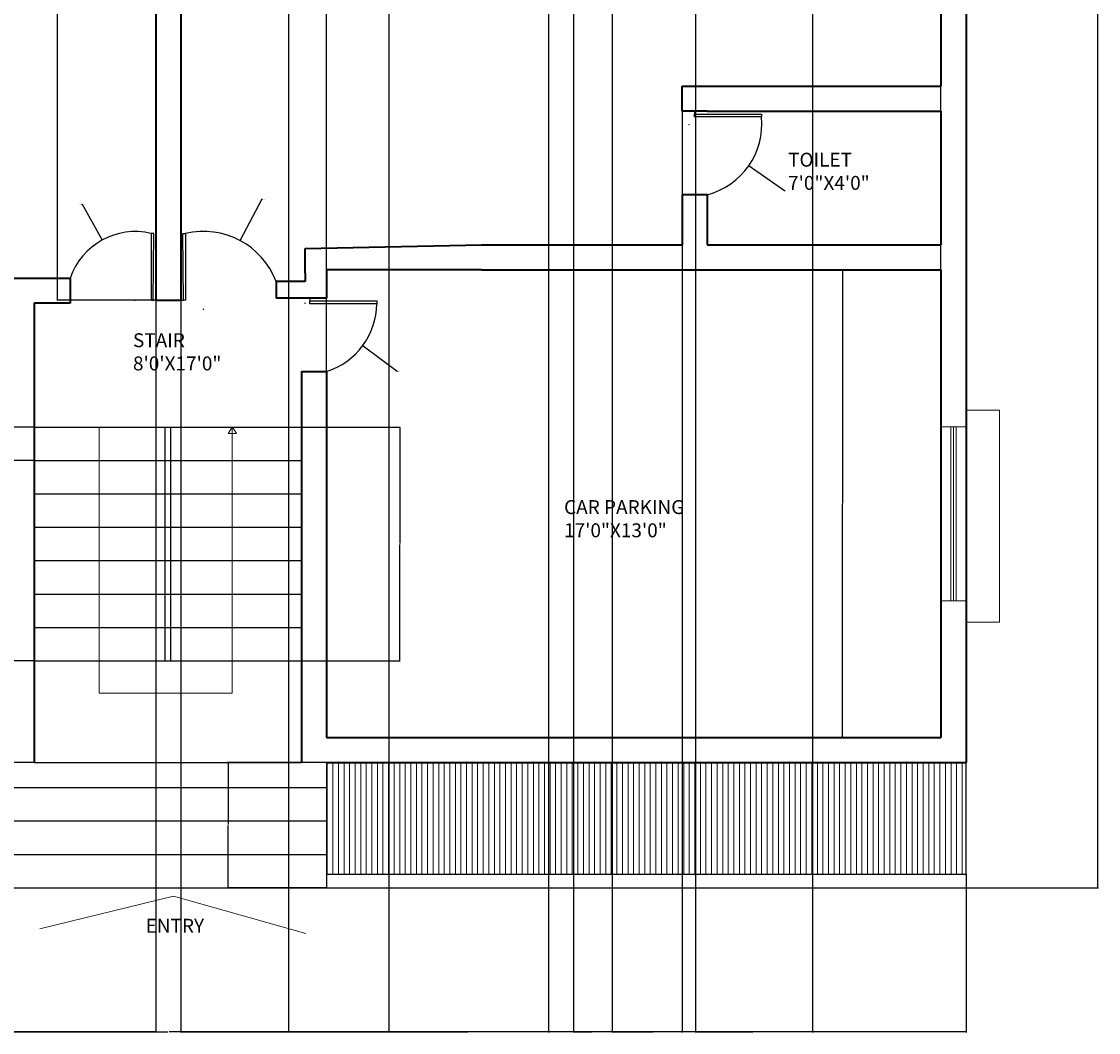
# Model space of a CAD drawing. Units: inches. Extents: x -35 to 633, y -653 to 119.
# Tile 2 of 4: x 246 to 633, y -653 to -289. Entities that reach past the tile are written whole.
import ezdxf

# ---------------------------------------------------------------- set-up
doc = ezdxf.new("R2010")
doc.units = ezdxf.units.IN
doc.header["$MEASUREMENT"] = 0
for name, color, linetype, lineweight in [('A-ANNO-DIMS', 2, 'Continuous', 18), ('A-ANNO-SYMB', 2, 'Continuous', 18), ('A-ANNO-TEXT', 7, 'Continuous', 25), ('A-AREA-IDEN', 7, 'Continuous', 18), ('A-DOOR', 3, 'Continuous', 25), ('A-FLOR-STRS', 7, 'Continuous', 25), ('A-GLAZ', 4, 'Continuous', 20), ('A-GLAZ-PROJ', 4, 'Continuous', 18), ('A-WALL', 7, 'Continuous', 35), ('L-HRDS', 8, 'Continuous', 25), ('L-HRDS-PATT', 252, 'Continuous', 13)]:
    doc.layers.add(name, color=color, linetype=linetype, lineweight=lineweight)
doc.styles.get("Standard").update_dxf_attribs({"font": 'arial.ttf'})
doc.dimstyles.get("Standard").update_dxf_attribs({"dimtxt": 0.18, "dimasz": 0.18, "dimexe": 0.18, "dimexo": 0.0625, "dimgap": 0.09, "dimtad": 0, "dimtih": 1, "dimtoh": 1, "dimdec": 4, "dimzin": 0, "dimdsep": 46, "dimtxsty": 'Standard', "dimcen": 0.09, "dimadec": 0, "dimazin": 0, "dimtfac": 1, "dimtdec": 4, "dimtofl": 0, "dimtmove": 0, "dimatfit": 3, "dimfxl": 1, "dimtolj": 1, "dimtzin": 0, "dimarcsym": 0})

# ---------------------------------------------------------------- blocks, each defined once
blk = doc.blocks.new('DOOR-LEAF-24IN')
for p, q in [((-1, 24), (-2, 24)), ((-2, 24), (-2, 0)), ((-1, 0), (-1, 24)), ((-2, 0), (-1, 0)), ((0, 0), (-1, 0))]:
    blk.add_line(p, q)
blk = doc.blocks.new('*D10')
at = {"layer": 'A-ANNO-DIMS', "color": 0, "lineweight": -2, "transparency": 16777216}
for p, q in [((12.69, -594.87), (12.69, -652.72)), ((585.69, -595.88), (585.69, -652.72)), ((12.87, -652.54), (298.9, -652.54)), ((585.51, -652.54), (299.48, -652.54))]:
    blk.add_line(p, q, dxfattribs=at)
at = {"layer": 'A-ANNO-DIMS', "color": 0, "transparency": 16777216}
for points in [[(12.87, -652.51), (12.87, -652.57), (12.69, -652.54)], [(585.51, -652.51), (585.51, -652.57), (585.69, -652.54)]]:
    blk.add_solid(points, dxfattribs=at)
at = {"layer": 'Defpoints', "color": 0, "transparency": 16777216}
for p in [(12.69, -594.81), (585.69, -595.82), (585.69, -652.54)]:
    blk.add_point(p, dxfattribs=at)
at = {"layer": 'A-ANNO-DIMS', "color": 0, "transparency": 16777216, "insert": (299.19, -652.54), "char_height": 0.18, "attachment_point": 5}
blk.add_mtext('\\A1;573', dxfattribs=at)
blk = doc.blocks.new('*D19')
at = {"layer": 'A-ANNO-DIMS', "color": 0, "lineweight": -2, "transparency": 16777216}
for p, q in [((303.69, 17.22), (303.69, -652.72)), ((342.39, 17.22), (342.39, -652.72)), ((303.87, -652.54), (322.57, -652.54)), ((342.21, -652.54), (323.5, -652.54))]:
    blk.add_line(p, q, dxfattribs=at)
at = {"layer": 'A-ANNO-DIMS', "color": 0, "transparency": 16777216}
for points in [[(303.87, -652.51), (303.87, -652.57), (303.69, -652.54)], [(342.21, -652.51), (342.21, -652.57), (342.39, -652.54)]]:
    blk.add_solid(points, dxfattribs=at)
at = {"layer": 'Defpoints', "color": 0, "transparency": 16777216}
for p in [(303.69, 17.29), (342.39, 17.29), (342.39, -652.54)]:
    blk.add_point(p, dxfattribs=at)
at = {"layer": 'A-ANNO-DIMS', "color": 0, "transparency": 16777216, "insert": (323.04, -652.54), "char_height": 0.18, "attachment_point": 5}
blk.add_mtext('\\A1;38.695', dxfattribs=at)
blk = doc.blocks.new('*D20')
at = {"layer": 'A-ANNO-DIMS', "color": 0, "lineweight": -2, "transparency": 16777216}
for p, q in [((378.39, 17.22), (378.39, -652.72)), ((435.69, 17.22), (435.69, -652.72)), ((378.57, -652.54), (406.71, -652.54)), ((435.51, -652.54), (407.36, -652.54))]:
    blk.add_line(p, q, dxfattribs=at)
at = {"layer": 'A-ANNO-DIMS', "color": 0, "transparency": 16777216}
for points in [[(378.57, -652.51), (378.57, -652.57), (378.39, -652.54)], [(435.51, -652.51), (435.51, -652.57), (435.69, -652.54)]]:
    blk.add_solid(points, dxfattribs=at)
at = {"layer": 'Defpoints', "color": 0, "transparency": 16777216}
for p in [(378.39, 17.29), (435.69, 17.29), (435.69, -652.54)]:
    blk.add_point(p, dxfattribs=at)
at = {"layer": 'A-ANNO-DIMS', "color": 0, "transparency": 16777216, "insert": (407.04, -652.54), "char_height": 0.18, "attachment_point": 5}
blk.add_mtext('\\A1;57.3', dxfattribs=at)
blk = doc.blocks.new('*D21')
at = {"layer": 'A-ANNO-DIMS', "color": 0, "lineweight": -2, "transparency": 16777216}
for p, q in [((444.69, 17.22), (444.69, -652.72)), ((458.58, 17.22), (458.58, -652.72)), ((444.87, -652.54), (451.25, -652.54)), ((458.4, -652.54), (452.02, -652.54))]:
    blk.add_line(p, q, dxfattribs=at)
at = {"layer": 'A-ANNO-DIMS', "color": 0, "transparency": 16777216}
for points in [[(444.87, -652.51), (444.87, -652.57), (444.69, -652.54)], [(458.4, -652.51), (458.4, -652.57), (458.58, -652.54)]]:
    blk.add_solid(points, dxfattribs=at)
at = {"layer": 'Defpoints', "color": 0, "transparency": 16777216}
for p in [(444.69, 17.29), (458.58, 17.29), (458.58, -652.54)]:
    blk.add_point(p, dxfattribs=at)
at = {"layer": 'A-ANNO-DIMS', "color": 0, "transparency": 16777216, "insert": (451.64, -652.54), "char_height": 0.18, "attachment_point": 5}
blk.add_mtext('\\A1;13.89', dxfattribs=at)
blk = doc.blocks.new('*D22')
at = {"layer": 'A-ANNO-DIMS', "color": 0, "lineweight": -2, "transparency": 16777216}
for p, q in [((458.58, 17.22), (458.58, -652.72)), ((488.58, 17.22), (488.58, -652.72)), ((458.76, -652.54), (473.36, -652.54)), ((488.4, -652.54), (473.8, -652.54))]:
    blk.add_line(p, q, dxfattribs=at)
at = {"layer": 'A-ANNO-DIMS', "color": 0, "transparency": 16777216}
for points in [[(458.76, -652.51), (458.76, -652.57), (458.58, -652.54)], [(488.4, -652.51), (488.4, -652.57), (488.58, -652.54)]]:
    blk.add_solid(points, dxfattribs=at)
at = {"layer": 'Defpoints', "color": 0, "transparency": 16777216}
for p in [(458.58, 17.29), (488.58, 17.29), (488.58, -652.54)]:
    blk.add_point(p, dxfattribs=at)
at = {"layer": 'A-ANNO-DIMS', "color": 0, "transparency": 16777216, "insert": (473.58, -652.54), "char_height": 0.18, "attachment_point": 5}
blk.add_mtext('\\A1;30', dxfattribs=at)
blk = doc.blocks.new('*D23')
at = {"layer": 'A-ANNO-DIMS', "color": 0, "lineweight": -2, "transparency": 16777216}
for p, q in [((488.58, 17.22), (488.58, -652.72)), ((530.49, 17.22), (530.49, -652.72)), ((488.76, -652.54), (509.15, -652.54)), ((530.31, -652.54), (509.91, -652.54))]:
    blk.add_line(p, q, dxfattribs=at)
at = {"layer": 'A-ANNO-DIMS', "color": 0, "transparency": 16777216}
for points in [[(488.76, -652.51), (488.76, -652.57), (488.58, -652.54)], [(530.31, -652.51), (530.31, -652.57), (530.49, -652.54)]]:
    blk.add_solid(points, dxfattribs=at)
at = {"layer": 'Defpoints', "color": 0, "transparency": 16777216}
for p in [(488.58, 17.29), (530.49, 17.29), (530.49, -652.54)]:
    blk.add_point(p, dxfattribs=at)
at = {"layer": 'A-ANNO-DIMS', "color": 0, "transparency": 16777216, "insert": (509.53, -652.54), "char_height": 0.18, "attachment_point": 5}
blk.add_mtext('\\A1;41.91', dxfattribs=at)
blk = doc.blocks.new('*D24')
at = {"layer": 'A-ANNO-DIMS', "color": 0, "lineweight": -2, "transparency": 16777216}
for p, q in [((585.75, 83.29), (633.22, 83.29)), ((633.04, 83.11), (633.04, -258.53)), ((633.04, -600.53), (633.04, -258.89)), ((356.04, -600.71), (633.22, -600.71))]:
    blk.add_line(p, q, dxfattribs=at)
at = {"layer": 'A-ANNO-DIMS', "color": 0, "transparency": 16777216}
for points in [[(633.01, 83.11), (633.07, 83.11), (633.04, 83.29)], [(633.01, -600.53), (633.07, -600.53), (633.04, -600.71)]]:
    blk.add_solid(points, dxfattribs=at)
at = {"layer": 'Defpoints', "color": 0, "transparency": 16777216}
for p in [(585.69, 83.29), (355.98, -600.71), (633.04, -600.71)]:
    blk.add_point(p, dxfattribs=at)
at = {"layer": 'A-ANNO-DIMS', "color": 0, "transparency": 16777216, "insert": (633.04, -258.71), "char_height": 0.18, "attachment_point": 5}
blk.add_mtext('\\A1;684', dxfattribs=at)
blk = doc.blocks.new('*D37')
at = {"layer": 'A-ANNO-DIMS', "color": 0, "lineweight": -2, "transparency": 16777216}
for p, q in [((355.98, -546.65), (355.98, 118.82)), ((356.16, 118.64), (465.94, 118.64)), ((576.51, 118.64), (466.73, 118.64)), ((576.69, -546.65), (576.69, 118.82))]:
    blk.add_line(p, q, dxfattribs=at)
at = {"layer": 'A-ANNO-DIMS', "color": 0, "transparency": 16777216}
for points in [[(356.16, 118.67), (356.16, 118.61), (355.98, 118.64)], [(576.51, 118.67), (576.51, 118.61), (576.69, 118.64)]]:
    blk.add_solid(points, dxfattribs=at)
at = {"layer": 'Defpoints', "color": 0, "transparency": 16777216}
for p in [(576.69, 118.64), (355.98, -546.71), (576.69, -546.71)]:
    blk.add_point(p, dxfattribs=at)
at = {"layer": 'A-ANNO-DIMS', "color": 0, "transparency": 16777216, "insert": (466.33, 118.64), "char_height": 0.18, "attachment_point": 5}
blk.add_mtext('\\A1;220.7', dxfattribs=at)
blk = doc.blocks.new('*D40')
at = {"layer": 'A-ANNO-DIMS', "color": 0, "lineweight": -2, "transparency": 16777216}
for p, q in [((576.63, -378.71), (541.16, -378.71)), ((541.34, -378.89), (541.34, -462.53)), ((541.34, -546.53), (541.34, -462.89)), ((576.63, -546.71), (541.16, -546.71))]:
    blk.add_line(p, q, dxfattribs=at)
at = {"layer": 'A-ANNO-DIMS', "color": 0, "transparency": 16777216}
for points in [[(541.31, -378.89), (541.37, -378.89), (541.34, -378.71)], [(541.31, -546.53), (541.37, -546.53), (541.34, -546.71)]]:
    blk.add_solid(points, dxfattribs=at)
at = {"layer": 'Defpoints', "color": 0, "transparency": 16777216}
for p in [(541.34, -378.71), (576.69, -378.71), (576.69, -546.71)]:
    blk.add_point(p, dxfattribs=at)
at = {"layer": 'A-ANNO-DIMS', "color": 0, "transparency": 16777216, "insert": (541.34, -462.71), "char_height": 0.18, "attachment_point": 5}
blk.add_mtext('\\A1;168', dxfattribs=at)
blk = doc.blocks.new('*D41')
at = {"layer": 'A-ANNO-DIMS', "color": 0, "lineweight": -2, "transparency": 16777216}
for p, q in [((347.04, -435.17), (382.51, -435.17)), ((382.33, -435.35), (382.33, -476.99)), ((382.33, -518.99), (382.33, -477.35)), ((347.04, -519.17), (382.51, -519.17))]:
    blk.add_line(p, q, dxfattribs=at)
at = {"layer": 'A-ANNO-DIMS', "color": 0, "transparency": 16777216}
for points in [[(382.3, -435.35), (382.36, -435.35), (382.33, -435.17)], [(382.3, -518.99), (382.36, -518.99), (382.33, -519.17)]]:
    blk.add_solid(points, dxfattribs=at)
at = {"layer": 'Defpoints', "color": 0, "transparency": 16777216}
for p in [(346.98, -435.17), (346.98, -519.17), (382.33, -519.17)]:
    blk.add_point(p, dxfattribs=at)
at = {"layer": 'A-ANNO-DIMS', "color": 0, "transparency": 16777216, "insert": (382.33, -477.17), "char_height": 0.18, "attachment_point": 5}
blk.add_mtext('\\A1;84', dxfattribs=at)
blk = doc.blocks.new('*D42')
at = {"layer": 'A-ANNO-DIMS', "color": 0, "lineweight": -2, "transparency": 16777216}
for p, q in [((250.91, -435.17), (215.45, -435.17)), ((215.63, -435.35), (215.63, -440.99)), ((215.63, -446.99), (215.63, -441.35)), ((250.91, -447.17), (215.45, -447.17))]:
    blk.add_line(p, q, dxfattribs=at)
at = {"layer": 'A-ANNO-DIMS', "color": 0, "transparency": 16777216}
for points in [[(215.6, -435.35), (215.66, -435.35), (215.63, -435.17)], [(215.6, -446.99), (215.66, -446.99), (215.63, -447.17)]]:
    blk.add_solid(points, dxfattribs=at)
at = {"layer": 'Defpoints', "color": 0, "transparency": 16777216}
for p in [(215.63, -435.17), (250.98, -435.17), (250.98, -447.17)]:
    blk.add_point(p, dxfattribs=at)
at = {"layer": 'A-ANNO-DIMS', "color": 0, "transparency": 16777216, "insert": (215.63, -441.17), "char_height": 0.18, "attachment_point": 5}
blk.add_mtext('\\A1;12', dxfattribs=at)
blk = doc.blocks.new('*D43')
at = {"layer": 'A-ANNO-DIMS', "color": 0, "lineweight": -2, "transparency": 16777216}
for p, q in [((250.91, -519.17), (215.45, -519.17)), ((215.63, -519.35), (215.63, -537.26)), ((215.63, -555.53), (215.63, -537.62)), ((250.91, -555.71), (215.45, -555.71))]:
    blk.add_line(p, q, dxfattribs=at)
at = {"layer": 'A-ANNO-DIMS', "color": 0, "transparency": 16777216}
for points in [[(215.6, -519.35), (215.66, -519.35), (215.63, -519.17)], [(215.6, -555.53), (215.66, -555.53), (215.63, -555.71)]]:
    blk.add_solid(points, dxfattribs=at)
at = {"layer": 'Defpoints', "color": 0, "transparency": 16777216}
for p in [(215.63, -519.17), (250.98, -519.17), (250.98, -555.71)]:
    blk.add_point(p, dxfattribs=at)
at = {"layer": 'A-ANNO-DIMS', "color": 0, "transparency": 16777216, "insert": (215.63, -537.44), "char_height": 0.18, "attachment_point": 5}
blk.add_mtext('\\A1;36.54', dxfattribs=at)
blk = doc.blocks.new('*D44')
at = {"layer": 'A-ANNO-DIMS', "color": 0, "lineweight": -2, "transparency": 16777216}
for p, q in [((355.91, -555.71), (320.45, -555.71)), ((320.63, -555.89), (320.63, -578.03)), ((320.63, -600.53), (320.63, -578.39)), ((355.91, -600.71), (320.45, -600.71))]:
    blk.add_line(p, q, dxfattribs=at)
at = {"layer": 'A-ANNO-DIMS', "color": 0, "transparency": 16777216}
for points in [[(320.6, -555.89), (320.66, -555.89), (320.63, -555.71)], [(320.6, -600.53), (320.66, -600.53), (320.63, -600.71)]]:
    blk.add_solid(points, dxfattribs=at)
at = {"layer": 'Defpoints', "color": 0, "transparency": 16777216}
for p in [(320.63, -555.71), (355.98, -555.71), (355.98, -600.71)]:
    blk.add_point(p, dxfattribs=at)
at = {"layer": 'A-ANNO-DIMS', "color": 0, "transparency": 16777216, "insert": (320.63, -578.21), "char_height": 0.18, "attachment_point": 5}
blk.add_mtext('\\A1;45', dxfattribs=at)
blk = doc.blocks.new('*D46')
at = {"layer": 'A-ANNO-DIMS', "color": 0, "lineweight": -2, "transparency": 16777216}
for p, q in [((294.63, -123.71), (259.16, -123.71)), ((259.34, -123.89), (259.34, -256.48)), ((259.34, -389.42), (259.34, -256.84)), ((294.63, -389.6), (259.16, -389.6))]:
    blk.add_line(p, q, dxfattribs=at)
at = {"layer": 'A-ANNO-DIMS', "color": 0, "transparency": 16777216}
for points in [[(259.31, -123.89), (259.37, -123.89), (259.34, -123.71)], [(259.31, -389.42), (259.37, -389.42), (259.34, -389.6)]]:
    blk.add_solid(points, dxfattribs=at)
at = {"layer": 'Defpoints', "color": 0, "transparency": 16777216}
for p in [(259.34, -123.71), (294.69, -123.71), (294.69, -389.6)]:
    blk.add_point(p, dxfattribs=at)
at = {"layer": 'A-ANNO-DIMS', "color": 0, "transparency": 16777216, "insert": (259.34, -256.66), "char_height": 0.18, "attachment_point": 5}
blk.add_mtext('\\A1;265.9', dxfattribs=at)
blk = doc.blocks.new('*D47')
at = {"layer": 'A-ANNO-DIMS', "color": 0, "lineweight": -2, "transparency": 16777216}
for p, q in [((294.69, -123.78), (294.69, -652.72)), ((126.69, -312.78), (126.69, -652.72)), ((126.87, -652.54), (210.41, -652.54)), ((294.51, -652.54), (210.97, -652.54))]:
    blk.add_line(p, q, dxfattribs=at)
at = {"layer": 'A-ANNO-DIMS', "color": 0, "transparency": 16777216}
for points in [[(126.87, -652.51), (126.87, -652.57), (126.69, -652.54)], [(294.51, -652.51), (294.51, -652.57), (294.69, -652.54)]]:
    blk.add_solid(points, dxfattribs=at)
at = {"layer": 'Defpoints', "color": 0, "transparency": 16777216}
for p in [(294.69, -123.71), (126.69, -312.71), (294.69, -652.54)]:
    blk.add_point(p, dxfattribs=at)
at = {"layer": 'A-ANNO-DIMS', "color": 0, "transparency": 16777216, "insert": (210.69, -652.54), "char_height": 0.18, "attachment_point": 5}
blk.add_mtext('\\A1;168', dxfattribs=at)
blk = doc.blocks.new('*D48')
at = {"layer": 'A-ANNO-DIMS', "color": 0, "lineweight": -2, "transparency": 16777216}
for p, q in [((303.69, -123.78), (303.69, -652.72)), ((483.69, -312.78), (483.69, -652.72)), ((303.87, -652.54), (393.41, -652.54)), ((483.51, -652.54), (393.97, -652.54))]:
    blk.add_line(p, q, dxfattribs=at)
at = {"layer": 'A-ANNO-DIMS', "color": 0, "transparency": 16777216}
for points in [[(303.87, -652.51), (303.87, -652.57), (303.69, -652.54)], [(483.51, -652.51), (483.51, -652.57), (483.69, -652.54)]]:
    blk.add_solid(points, dxfattribs=at)
at = {"layer": 'Defpoints', "color": 0, "transparency": 16777216}
for p in [(303.69, -123.71), (483.69, -312.71), (483.69, -652.54)]:
    blk.add_point(p, dxfattribs=at)
at = {"layer": 'A-ANNO-DIMS', "color": 0, "transparency": 16777216, "insert": (393.69, -652.54), "char_height": 0.18, "attachment_point": 5}
blk.add_mtext('\\A1;180', dxfattribs=at)
blk = doc.blocks.new('*D54')
at = {"layer": 'A-ANNO-DIMS', "color": 0, "lineweight": -2, "transparency": 16777216}
for p, q in [((332.74, -353.35), (324.98, -367.99)), ((332.92, -353.35), (332.74, -353.35)), ((311.71, -392.81), (311.89, -392.81)), ((311.8, -392.9), (311.8, -392.72))]:
    blk.add_line(p, q, dxfattribs=at)
at = {"layer": 'A-ANNO-DIMS', "color": 0, "transparency": 16777216}
blk.add_solid([(324.95, -367.97), (325, -368), (324.89, -368.15)], dxfattribs=at)
at = {"layer": 'Defpoints', "color": 0, "transparency": 16777216}
for p in [(324.89, -368.15), (311.8, -392.81)]:
    blk.add_point(p, dxfattribs=at)
at = {"layer": 'A-ANNO-DIMS', "color": 0, "transparency": 16777216, "insert": (333.4, -353.35), "char_height": 0.18, "attachment_point": 5}
blk.add_mtext('\\A1;R27.92', dxfattribs=at)
blk = doc.blocks.new('*D56')
at = {"layer": 'A-ANNO-DIMS', "color": 0, "lineweight": -2, "transparency": 16777216}
for p, q in [((486.12, -326.41), (486.3, -326.41)), ((486.21, -326.5), (486.21, -326.32)), ((520.51, -350.29), (507.79, -341.44)), ((520.69, -350.29), (520.51, -350.29))]:
    blk.add_line(p, q, dxfattribs=at)
at = {"layer": 'A-ANNO-DIMS', "color": 0, "transparency": 16777216}
blk.add_solid([(507.81, -341.41), (507.77, -341.46), (507.64, -341.34)], dxfattribs=at)
at = {"layer": 'Defpoints', "color": 0, "transparency": 16777216}
for p in [(486.21, -326.41), (507.64, -341.34)]:
    blk.add_point(p, dxfattribs=at)
at = {"layer": 'A-ANNO-DIMS', "color": 0, "transparency": 16777216, "insert": (521.24, -350.29), "char_height": 0.18, "attachment_point": 5}
blk.add_mtext('\\A1;R26.125', dxfattribs=at)
blk = doc.blocks.new('*D57')
at = {"layer": 'A-ANNO-DIMS', "color": 0, "lineweight": -2, "transparency": 16777216}
for p, q in [((348.35, -390.76), (348.35, -390.58)), ((348.26, -390.67), (348.44, -390.67)), ((381.36, -415.19), (369.13, -406.11)), ((381.54, -415.19), (381.36, -415.19))]:
    blk.add_line(p, q, dxfattribs=at)
at = {"layer": 'A-ANNO-DIMS', "color": 0, "transparency": 16777216}
blk.add_solid([(369.15, -406.08), (369.11, -406.13), (368.98, -406)], dxfattribs=at)
at = {"layer": 'Defpoints', "color": 0, "transparency": 16777216}
for p in [(348.35, -390.67), (368.98, -406)]:
    blk.add_point(p, dxfattribs=at)
at = {"layer": 'A-ANNO-DIMS', "color": 0, "transparency": 16777216, "insert": (381.95, -415.19), "char_height": 0.18, "attachment_point": 5}
blk.add_mtext('\\A1;R25.7', dxfattribs=at)
blk = doc.blocks.new('*D59')
at = {"layer": 'A-ANNO-DIMS', "color": 0, "lineweight": -2, "transparency": 16777216}
for p, q in [((268.03, -355.09), (268.21, -355.09)), ((268.21, -355.09), (275.28, -367.85)), ((287.21, -389.55), (287.39, -389.55)), ((287.3, -389.64), (287.3, -389.46))]:
    blk.add_line(p, q, dxfattribs=at)
at = {"layer": 'A-ANNO-DIMS', "color": 0, "transparency": 16777216}
blk.add_solid([(275.31, -367.84), (275.26, -367.87), (275.37, -368.01)], dxfattribs=at)
at = {"layer": 'Defpoints', "color": 0, "transparency": 16777216}
for p in [(275.37, -368.01), (287.3, -389.55)]:
    blk.add_point(p, dxfattribs=at)
at = {"layer": 'A-ANNO-DIMS', "color": 0, "transparency": 16777216, "insert": (267.55, -355.09), "char_height": 0.18, "attachment_point": 5}
blk.add_mtext('\\A1;R24.62', dxfattribs=at)

msp = doc.modelspace()

# ---------------------------------------------------------------- hatches: boundary and pattern name
at = {"layer": 'L-HRDS-PATT'}
h = msp.add_hatch(dxfattribs=at)
h.set_pattern_fill('ANSI31', color=256, scale=16, angle=45, style=0)
h.set_pattern_definition([(90, (-2179.7136, -1471.1113), (-2, 0), [])])
h.paths.add_polyline_path([(355.9768, -595.8152), (585.6907, -595.8152), (585.6907, -555.713), (355.9768, -555.713)])

# ---------------------------------------------------------------- linework, layer by layer
at = {"layer": 'A-ANNO-SYMB'}
for p, q in [((274.3662, -435.1709), (274.3662, -530.8377)), ((322.0837, -435.1709), (320.7222, -437.529)), ((322.0837, -530.8377), (322.0837, -435.1709)), ((323.6397, -437.529), (322.2782, -435.1709)), ((320.7222, -437.529), (323.6397, -437.529)), ((274.3662, -530.8377), (322.0837, -530.8377)), ((301.0168, -603.7011), (253.0683, -615.458)), ((301.0168, -603.7011), (348.619, -617.187))]:
    msp.add_line(p, q, dxfattribs=at)
at = {"layer": 'A-DOOR'}
for p, q in [((294.0401, -365.606), (293.0401, -365.606)), ((293.0401, -365.606), (293.0401, -389.606)), ((293.6907, -389.6034), (294.0401, -365.606)), ((304.69, -389.6389), (304.3725, -365.641)), ((304.3725, -365.641), (305.3725, -365.641)), ((305.3725, -365.641), (305.3725, -389.641)), ((293.0401, -389.606), (294.0401, -389.606)), ((294.6907, -389.6034), (293.6907, -389.6034)), ((303.6907, -389.6034), (304.69, -389.6389)), ((305.3725, -389.641), (304.3725, -389.641))]:
    msp.add_line(p, q, dxfattribs=at)
for centre, radius, start, end in [((486.2053, -326.4062), 26.1246, 284.373894, 5.917194), ((287.2987, -389.5486), 24.6214, 76.515385, 161.44307), ((311.8045, -392.8103), 27.9203, 20.775692, 103.319004), ((348.3486, -390.6748), 25.7021, 287.265117, 359.542731)]:
    msp.add_arc(centre, radius, start, end, dxfattribs=at)
at = {"layer": 'A-FLOR-STRS'}
for p, q in [((250.9768, -435.1709), (346.9768, -435.1709)), ((297.9768, -435.1709), (297.9768, -519.1709)), ((299.9768, -435.1709), (299.9768, -519.1709)), ((250.9768, -447.1709), (346.9768, -447.1709)), ((250.9768, -459.1709), (346.9768, -459.1709)), ((250.9768, -471.1709), (346.9768, -471.1709)), ((250.9768, -483.1709), (346.9768, -483.1709)), ((250.9768, -495.1709), (346.9768, -495.1709)), ((250.9768, -507.1709), (346.9768, -507.1709)), ((250.9768, -507.1709), (346.9768, -507.1709)), ((250.9768, -519.1709), (346.9768, -519.1709)), ((250.9768, -555.713), (346.9768, -555.713)), ((355.9768, -555.713), (355.9768, -564.713)), ((241.9768, -564.713), (355.9768, -564.713)), ((355.9768, -564.713), (355.9768, -600.713)), ((241.9768, -576.713), (355.9768, -576.713)), ((241.9768, -588.713), (355.9768, -588.713)), ((241.9768, -600.713), (355.9768, -600.713)), ((254.4542, -600.713), (339.8944, -600.713))]:
    msp.add_line(p, q, dxfattribs=at)
at = {"layer": 'A-GLAZ'}
for p, q in [((576.6907, -435.0596), (585.6907, -435.0596)), ((580.1907, -435.0596), (580.1907, -497.5918)), ((581.1907, -435.0596), (581.1907, -497.5918)), ((582.1907, -435.0596), (582.1907, -497.5918)), ((576.6907, -497.5918), (585.6907, -497.5918))]:
    msp.add_line(p, q, dxfattribs=at)
at = {"layer": 'A-GLAZ-PROJ'}
for p, q in [((585.6907, -429.0928), (597.6907, -429.0928)), ((597.6907, -429.0928), (597.6907, -505.268)), ((597.6907, -505.268), (585.6907, -505.268))]:
    msp.add_line(p, q, dxfattribs=at)
at = {"layer": 'A-WALL'}
for p, q in [((585.6907, -114.713), (585.6907, -555.713)), ((294.6907, -123.713), (294.6907, -389.6034)), ((303.6907, -123.713), (303.6907, -389.6034)), ((576.6907, -180.713), (576.6907, -312.713)), ((483.6907, -312.713), (576.6907, -312.713)), ((483.6907, -321.713), (483.6907, -312.713)), ((492.6907, -321.713), (483.6907, -321.713)), ((492.6907, -321.713), (576.6907, -321.713)), ((576.6907, -321.713), (576.6907, -369.713)), ((483.6907, -351.713), (483.6907, -369.713)), ((492.6907, -351.713), (483.6907, -351.713)), ((492.6907, -351.713), (492.6907, -369.713)), ((348.3577, -370.9894), (411.6907, -369.713)), ((348.3577, -379.9347), (348.3577, -370.9894)), ((411.6907, -369.713), (483.6907, -369.713)), ((492.6907, -369.713), (576.6907, -369.713)), ((411.6907, -378.713), (355.9768, -378.713)), ((355.9768, -378.713), (355.9768, -388.88)), ((411.6907, -378.713), (576.6907, -378.713)), ((576.6907, -378.713), (576.6907, -546.713)), ((241.9768, -381.713), (250.9768, -381.713)), ((250.9768, -381.713), (263.9575, -381.713)), ((263.9575, -381.713), (263.9575, -390.713)), ((348.3577, -379.9347), (348.3577, -382.9067)), ((348.3577, -382.9067), (337.9094, -382.9067)), ((337.9094, -382.9067), (337.9094, -388.88)), ((294.6907, -389.6034), (303.6907, -389.6034)), ((355.9768, -388.88), (337.9094, -388.88)), ((250.9768, -390.713), (250.9768, -555.713)), ((263.9575, -390.713), (250.9768, -390.713)), ((346.9768, -415.2188), (346.9768, -555.713)), ((346.9768, -415.2188), (355.9768, -415.2188)), ((355.9768, -415.2188), (355.9768, -546.713)), ((355.9768, -546.713), (411.6907, -546.713)), ((411.6907, -546.713), (576.6907, -546.713)), ((355.9768, -555.713), (585.6907, -555.713))]:
    msp.add_line(p, q, dxfattribs=at)
at = {"layer": 'L-HRDS'}
for p, q in [((585.6907, -595.8152), (585.6907, -555.713)), ((355.9768, -595.8152), (585.6907, -595.8152))]:
    msp.add_line(p, q, dxfattribs=at)

# ---------------------------------------------------------------- block references
at = {"layer": 'A-DOOR', "extrusion": (0, 0, -1), "zscale": -1}
for p, rotation in [((-488.1907, -321.713), 89.99999999999999), ((-350.0498, -388.88), 90.00000000000003)]:
    msp.add_blockref('DOOR-LEAF-24IN', p, dxfattribs=dict(at, rotation=rotation))

# ---------------------------------------------------------------- texts
at = {"layer": 'A-ANNO-TEXT', "insert": (291.0525, -611.8649), "char_height": 5, "attachment_point": 1}
msp.add_mtext_dynamic_manual_height_columns('ENTRY', width=25.222092, gutter_width=25, heights=[0], dxfattribs=at)
at = {"layer": 'A-AREA-IDEN', "char_height": 5, "attachment_point": 1}
for s, width, insert in [('TOILET\\P7\'0"X4\'0"', 36.076101, (521.7779, -336.6165)), ('STAIR\\P8\'0\'X17\'0"', 41.424204, (286.4952, -401.4872)), ('CAR PARKING\\P17\'0"X13\'0"', 89.571033, (441.318, -461.447))]:
    msp.add_mtext_dynamic_manual_height_columns(s, width=width, gutter_width=25, heights=[0], dxfattribs=dict(at, insert=insert))

# ---------------------------------------------------------------- dimensions: what is measured, and where the dimension line sits
at = {"layer": 'A-ANNO-DIMS'}
for base, p1, p2, override, picture, middle in [((576.6907, 118.637), (355.9768, -546.713), (576.6907, -546.713), {"dimdec": 1, "dimlfac": 1, "dimrnd": 0, "dimzin": 0, "dimdsep": 46, "dimlunit": 2}, '*D37', (466.3337, 118.637)), ((342.3856, -652.537), (303.6907, 17.287), (342.3856, 17.287), {"dimdec": 3, "dimlfac": 1, "dimrnd": 0, "dimzin": 0, "dimdsep": 46, "dimlunit": 2}, '*D19', (323.0381, -652.537)), ((435.6907, -652.537), (378.3856, 17.287), (435.6907, 17.287), {"dimdec": 1, "dimlfac": 1, "dimrnd": 0, "dimzin": 0, "dimdsep": 46, "dimlunit": 2}, '*D20', (407.0381, -652.537)), ((458.5795, -652.537), (444.6907, 17.287), (458.5795, 17.287), {"dimdec": 2, "dimlfac": 1, "dimrnd": 0, "dimzin": 0, "dimdsep": 46, "dimlunit": 2}, '*D21', (451.6351, -652.537)), ((488.5795, -652.537), (458.5795, 17.287), (488.5795, 17.287), {"dimdec": 0, "dimlfac": 1, "dimrnd": 0, "dimzin": 0, "dimdsep": 46, "dimlunit": 2}, '*D22', (473.5795, -652.537)), ((530.4897, -652.537), (488.5795, 17.287), (530.4897, 17.287), {"dimdec": 2, "dimlfac": 1, "dimrnd": 0, "dimzin": 0, "dimdsep": 46, "dimlunit": 2}, '*D23', (509.5346, -652.537)), ((294.6907, -652.537), (126.6907, -312.713), (294.6907, -123.713), {"dimdec": 0, "dimlfac": 1, "dimrnd": 0, "dimzin": 0, "dimdsep": 46, "dimlunit": 2}, '*D47', (210.6907, -652.537)), ((483.6907, -652.537), (303.6907, -123.713), (483.6907, -312.713), {"dimdec": 0, "dimlfac": 1, "dimrnd": 0, "dimzin": 0, "dimdsep": 46, "dimlunit": 2}, '*D48', (393.6907, -652.537)), ((585.6907, -652.537), (12.6907, -594.812), (585.6907, -595.8152), {"dimdec": 0, "dimlfac": 1, "dimrnd": 0, "dimzin": 0, "dimdsep": 46, "dimlunit": 2}, '*D10', (299.1907, -652.537))]:
    dim = msp.add_linear_dim(base=base, p1=p1, p2=p2, dimstyle='Standard', override=override, dxfattribs=at)
    dim.commit()
    dim.dimension.update_dxf_attribs({"geometry": picture, "text_midpoint": middle})
for base, p1, p2, angle, override, picture, middle in [((633.0407, -600.713), (585.6907, 83.287), (355.9768, -600.713), 90, {"dimdec": 0, "dimlfac": 1, "dimrnd": 0, "dimzin": 0, "dimdsep": 46, "dimlunit": 2}, '*D24', (633.0407, -258.713)), ((259.3407, -123.713), (294.6907, -389.6034), (294.6907, -123.713), 90, {"dimdec": 1, "dimlfac": 1, "dimrnd": 0, "dimzin": 0, "dimdsep": 46, "dimlunit": 2}, '*D46', (259.3407, -256.6582)), ((541.3407, -378.713), (576.6907, -546.713), (576.6907, -378.713), 90, {"dimdec": 0, "dimlfac": 1, "dimrnd": 0, "dimzin": 0, "dimdsep": 46, "dimlunit": 2}, '*D40', (541.3407, -462.713)), ((215.6268, -435.1709), (250.9768, -447.1709), (250.9768, -435.1709), 90, {"dimdec": 0, "dimlfac": 1, "dimrnd": 0, "dimzin": 0, "dimdsep": 46, "dimlunit": 2}, '*D42', (215.6268, -441.1709)), ((382.3268, -519.1709), (346.9768, -435.1709), (346.9768, -519.1709), 270, {"dimdec": 0, "dimlfac": 1, "dimrnd": 0, "dimzin": 0, "dimdsep": 46, "dimlunit": 2}, '*D41', (382.3268, -477.1709)), ((215.6268, -519.1709), (250.9768, -555.713), (250.9768, -519.1709), 90, {"dimdec": 2, "dimlfac": 1, "dimrnd": 0, "dimzin": 0, "dimdsep": 46, "dimlunit": 2}, '*D43', (215.6268, -537.4419)), ((320.6268, -555.713), (355.9768, -600.713), (355.9768, -555.713), 90, {"dimdec": 0, "dimlfac": 1, "dimrnd": 0, "dimzin": 0, "dimdsep": 46, "dimlunit": 2}, '*D44', (320.6268, -578.213))]:
    dim = msp.add_linear_dim(base=base, p1=p1, p2=p2, angle=angle, dimstyle='Standard', override=override, dxfattribs=at)
    dim.commit()
    dim.dimension.update_dxf_attribs({"geometry": picture, "text_midpoint": middle})
for center, mpoint, override, picture, middle in [((486.2053, -326.4062), (507.6433, -341.3362), {"dimdec": 3, "dimlfac": 1, "dimrnd": 0, "dimzin": 0, "dimdsep": 46, "dimlunit": 2}, '*D56', (521.2365, -350.2942)), ((287.2987, -389.5486), (275.3699, -368.0099), {"dimdec": 2, "dimlfac": 1, "dimrnd": 0, "dimzin": 0, "dimdsep": 46, "dimlunit": 2}, '*D59', (267.5538, -355.0867)), ((311.8045, -392.8103), (324.8919, -368.1473), {"dimdec": 2, "dimlfac": 1, "dimrnd": 0, "dimzin": 0, "dimdsep": 46, "dimlunit": 2}, '*D54', (333.4032, -353.3494)), ((348.3486, -390.6748), (368.9836, -405.9977), {"dimdec": 1, "dimlfac": 1, "dimrnd": 0, "dimzin": 0, "dimdsep": 46, "dimlunit": 2}, '*D57', (381.9546, -415.1915))]:
    dim = msp.add_radius_dim(center=center, mpoint=mpoint, dimstyle='Standard', override=override, dxfattribs=at)
    dim.commit()
    dim.dimension.update_dxf_attribs({"geometry": picture, "text_midpoint": middle, "dimtype": 164})

doc.saveas('drawing.dxf')
